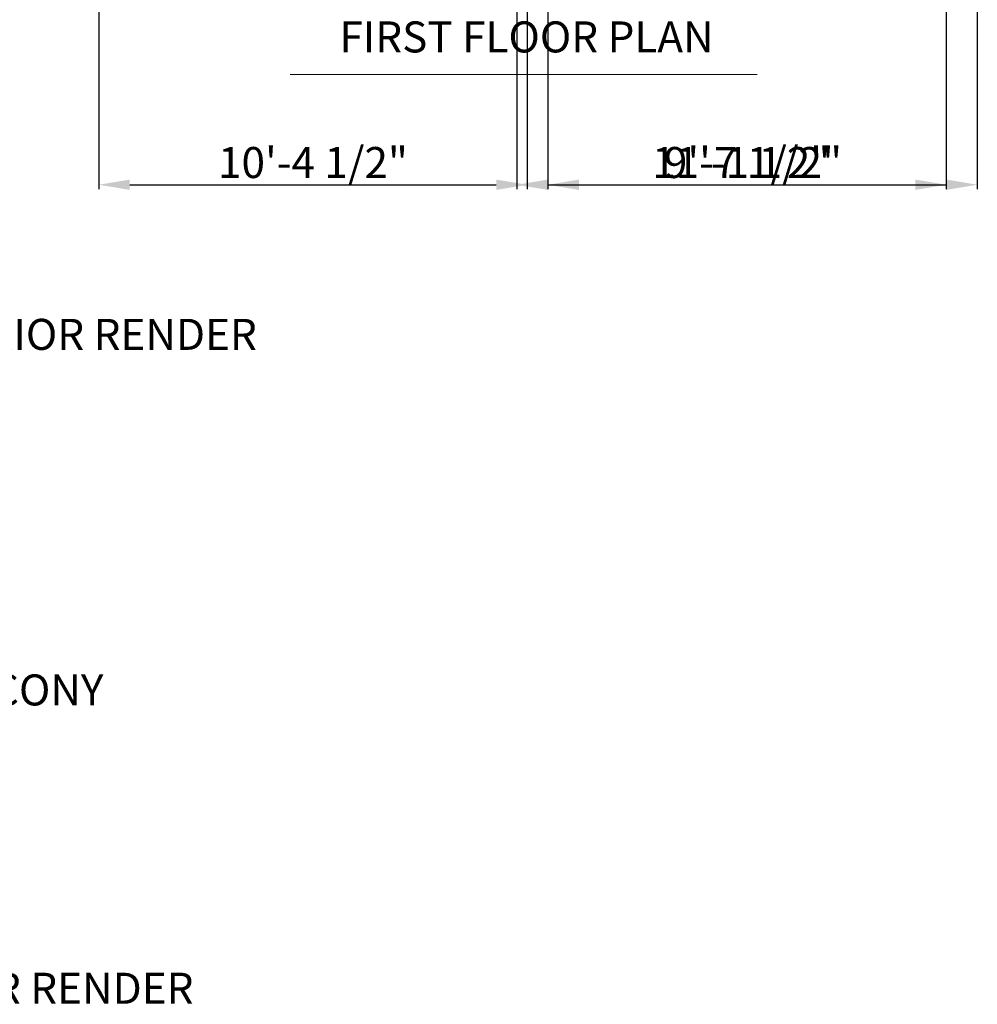
# Model space of a CAD drawing. Units: inches. Extents: x 2429 to 3343, y 1496 to 2530.
# Tile 2 of 7: x 2991 to 3269, y 1624 to 1910. Entities that reach past the tile are written whole.
import ezdxf

# ---------------------------------------------------------------- set-up
doc = ezdxf.new("R2010")
doc.units = ezdxf.units.IN
doc.layers.add('A-ANNO-DIMS', color=2, linetype='Continuous', lineweight=18)
doc.layers.add('A-ANNO-TEXT', color=7, linetype='Continuous', lineweight=18)
doc.styles.get("Standard").update_dxf_attribs({"font": 'arial.ttf'})
doc.dimstyles.new('ISO-25', dxfattribs={"dimtxt": 9, "dimasz": 9, "dimexe": 1.25, "dimexo": 0.625, "dimtad": 1, "dimdec": 1, "dimlunit": 3, "dimtxsty": 'Standard', "dimcen": 9, "dimadec": 0, "dimazin": 0, "dimtfac": 1, "dimtdec": 1, "dimtmove": 0, "dimatfit": 3, "dimfxl": 1, "dimarcsym": 0})

# ---------------------------------------------------------------- blocks, each defined once
blk = doc.blocks.new('*D65')
at = {"layer": 'A-ANNO-DIMS', "color": 0, "lineweight": -2, "transparency": 16777216}
for p, q in [((3014.05, 2027.16), (3014.05, 1860.42)), ((3138.41, 2027.16), (3138.41, 1860.42)), ((3023.05, 1861.67), (3129.41, 1861.67))]:
    blk.add_line(p, q, dxfattribs=at)
at = {"layer": 'A-ANNO-DIMS', "color": 0, "transparency": 16777216}
for points in [[(3023.05, 1863.17), (3023.05, 1860.17), (3014.05, 1861.67)], [(3129.41, 1863.17), (3129.41, 1860.17), (3138.41, 1861.67)]]:
    blk.add_solid(points, dxfattribs=at)
at = {"layer": 'Defpoints', "color": 0, "transparency": 16777216}
for p in [(3014.05, 2027.79), (3138.41, 2027.79), (3138.41, 1861.67)]:
    blk.add_point(p, dxfattribs=at)
at = {"layer": 'A-ANNO-DIMS', "color": 0, "transparency": 16777216, "insert": (3076.23, 1866.95), "char_height": 9, "attachment_point": 5}
blk.add_mtext('10\'-4 1/2"', dxfattribs=at)
blk = doc.blocks.new('*D67')
at = {"layer": 'A-ANNO-DIMS', "color": 0, "lineweight": -2, "transparency": 16777216}
for p, q in [((3144.41, 2027.16), (3144.41, 1860.42)), ((3260.05, 2027.16), (3260.05, 1860.42)), ((3153.41, 1861.67), (3251.05, 1861.67))]:
    blk.add_line(p, q, dxfattribs=at)
at = {"layer": 'A-ANNO-DIMS', "color": 0, "transparency": 16777216}
for points in [[(3153.41, 1863.17), (3153.41, 1860.17), (3144.41, 1861.67)], [(3251.05, 1863.17), (3251.05, 1860.17), (3260.05, 1861.67)]]:
    blk.add_solid(points, dxfattribs=at)
at = {"layer": 'Defpoints', "color": 0, "transparency": 16777216}
for p in [(3144.41, 2027.79), (3260.05, 2027.79), (3260.05, 1861.67)]:
    blk.add_point(p, dxfattribs=at)
at = {"layer": 'A-ANNO-DIMS', "color": 0, "transparency": 16777216, "insert": (3202.23, 1866.95), "char_height": 9, "attachment_point": 5}
blk.add_mtext('9\'-7 1/2"', dxfattribs=at)
blk = doc.blocks.new('*D70')
at = {"layer": 'A-ANNO-DIMS', "color": 0, "lineweight": -2, "transparency": 16777216}
for p, q in [((3135.41, 1969.85), (3135.41, 1860.42)), ((3269.05, 1969.85), (3269.05, 1860.42)), ((3144.41, 1861.67), (3260.05, 1861.67))]:
    blk.add_line(p, q, dxfattribs=at)
at = {"layer": 'A-ANNO-DIMS', "color": 0, "transparency": 16777216}
for points in [[(3144.41, 1863.17), (3144.41, 1860.17), (3135.41, 1861.67)], [(3260.05, 1863.17), (3260.05, 1860.17), (3269.05, 1861.67)]]:
    blk.add_solid(points, dxfattribs=at)
at = {"layer": 'Defpoints', "color": 0, "transparency": 16777216}
for p in [(3135.41, 1970.47), (3269.05, 1970.47), (3269.05, 1861.67)]:
    blk.add_point(p, dxfattribs=at)
at = {"layer": 'A-ANNO-DIMS', "color": 0, "transparency": 16777216, "insert": (3202.23, 1866.95), "char_height": 9, "attachment_point": 5}
blk.add_mtext('11\'-1 1/2"', dxfattribs=at)

msp = doc.modelspace()

# ---------------------------------------------------------------- linework, layer by layer
at = {"layer": 'A-ANNO-TEXT'}
msp.add_line((3069.58839, 1893.66916), (3205.11652, 1893.66916), dxfattribs=at)

# ---------------------------------------------------------------- texts
at = {"layer": 'A-ANNO-TEXT', "char_height": 9, "attachment_point": 1}
for s, width, insert in [('{\\fCalibri|b0|i0|c0|p34;FIRST FLOOR PLAN}', 127.7266644, (3083.92522, 1909.06231)), ('{\\fCalibri|b0|i0|c0|p34;EXTERIOR RENDER}', 142.5053551, (2952.63942, 1822.751)), ('{\\fCalibri|b0|i0|c0|p34;SIMPLE BALCONY RAILING}', 142.5053551, (2915.5451, 1719.56551)), ('{\\fCalibri|b0|i0|c0|p34;EXTERIOR RENDER}', 142.5053551, (2934.25813, 1633.00794))]:
    msp.add_mtext_dynamic_manual_height_columns(s, width=width, gutter_width=12.5, heights=[0], dxfattribs=dict(at, insert=insert))

# ---------------------------------------------------------------- dimensions: what is measured, and where the dimension line sits
at = {"layer": 'A-ANNO-DIMS'}
for base, p1, p2, picture, middle in [((3138.41055, 1861.66916), (3014.04839, 2027.78649), (3138.41055, 2027.78649), '*D65', (3076.22947, 1866.94764)), ((3260.04839, 1861.66916), (3144.41055, 2027.78649), (3260.04839, 2027.78649), '*D67', (3202.22947, 1866.94764)), ((3269.04839, 1861.66916), (3135.41055, 1970.47184), (3269.04839, 1970.47184), '*D70', (3202.22947, 1866.94764))]:
    dim = msp.add_linear_dim(base=base, p1=p1, p2=p2, dimstyle='ISO-25', override={"dimdec": 1, "dimlfac": 1, "dimrnd": 0, "dimzin": 1, "dimdsep": 46, "dimlunit": 4, "dimfrac": 2}, dxfattribs=at)
    dim.commit()
    dim.dimension.update_dxf_attribs({"geometry": picture, "text_midpoint": middle})

doc.saveas('drawing.dxf')
